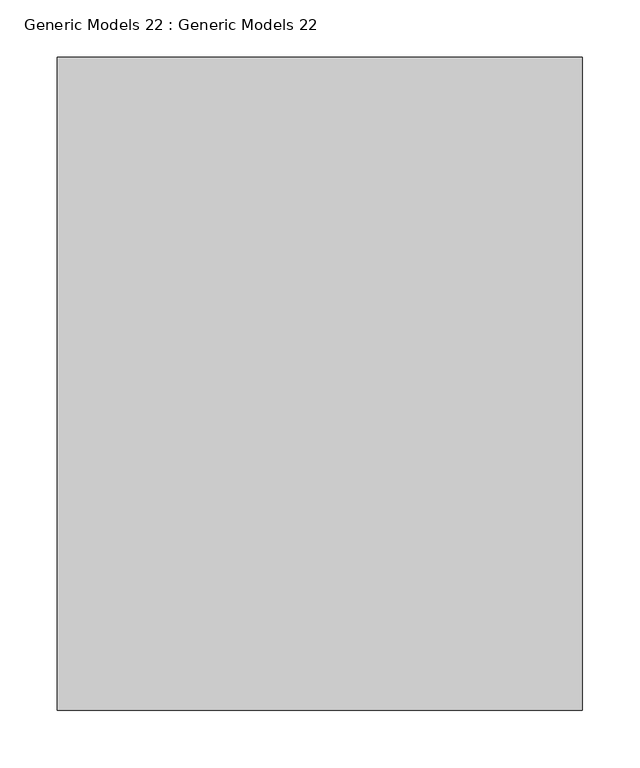
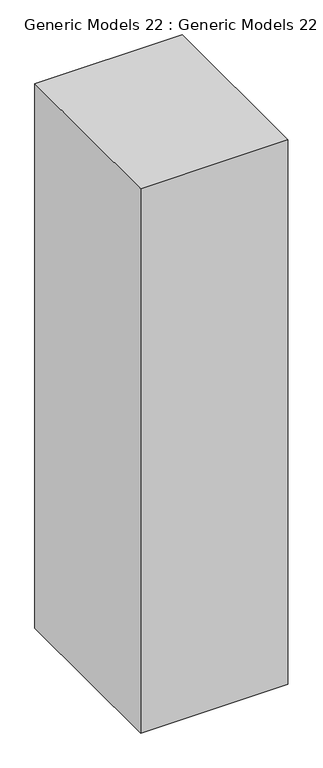
"""IFC4 building model written with IfcOpenShell, lengths in millimetres: proxy geometry, Generic Models 22 : Generic Models 22."""

from ifc_helpers import new_model, si_unit, frame, origin, place, context, project, spatial, polyline, outline, extrude, source, transform, mapped, element, save


def generic_models_22_generic_models_22_43b51bfc(model_context):
    return source(origin(), model_context, "Body", "SweptSolid", [
        extrude(outline(polyline([(-8443.9263881, -7819.7402622), (-8443.9263881, -8388.4150903), (-8901.1263881, -8388.4150903), (-8901.1263881, -7819.7402622), (-8443.9263881, -7819.7402622)])), frame((0.0, 0.0, 6748.0548819), z_axis=(0.0, 0.0, 1.0), x_axis=(1.0, 0.0, 0.0)), (0.0, 0.0, 1.0), 1786.3451181),
    ])


if __name__ == "__main__":
    model = new_model("IFC4")
    model_context = context("Model", 3, world=origin())
    ifc_project = project(units=[si_unit("LENGTHUNIT", "METRE", prefix="MILLI")], contexts=[model_context])
    site = spatial("IfcSite", under=ifc_project)
    building = spatial("IfcBuilding", under=site)
    placement = place(None, origin())
    generic_models_22_generic_models_22_shape = generic_models_22_generic_models_22_43b51bfc(model_context)
    element("IfcBuildingElementProxy", 1, Name="Generic Models 22 : Generic Models 22", ObjectType="Generic Models 22 : Generic Models 22", at=placement, inside=building, context=model_context, shape_type="MappedRepresentation", body=[
        mapped(generic_models_22_generic_models_22_shape, transform((0.0, 0.0, 0.0), x_axis=(1.0, 0.0, 0.0), y_axis=(0.0, 1.0, 0.0), z_axis=(0.0, 0.0, 1.0))),
    ])
    save(model, "model.ifc")

# Revit data of these elements
# Element 1 (IfcBuildingElementProxy, "Generic Models 22 : Generic Models 22")
#   Materials on its faces: "ESPRESSO"
# Materials
#   "ESPRESSO": class "Generic", colour RGB 120 120 120, transparency 0, Cost = 0
